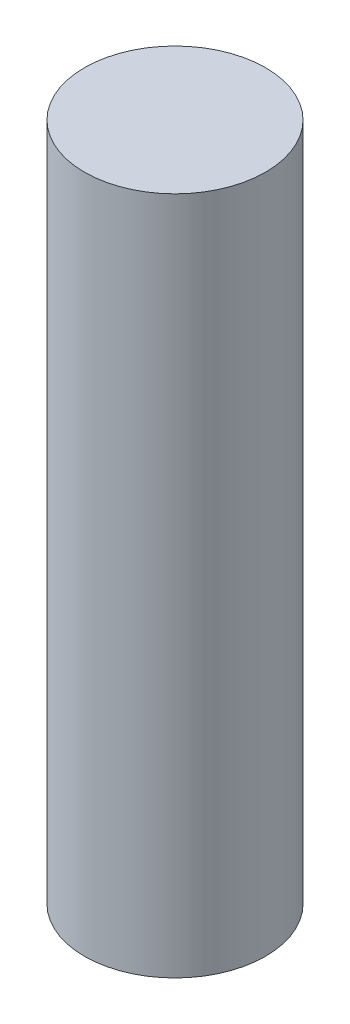
ISO-10303-21;
HEADER;
FILE_DESCRIPTION(('STEP AP214'),'2;1');
FILE_NAME('part.step','',(''),(''),'','','');
FILE_SCHEMA(('AUTOMOTIVE_DESIGN { 1 0 10303 214 1 1 1 1 }'));
ENDSEC;
DATA;
#1=APPLICATION_CONTEXT('core data for automotive mechanical design processes');
#2=APPLICATION_PROTOCOL_DEFINITION('international standard','automotive_design',2000,#1);
#3=PRODUCT_CONTEXT('',#1,'mechanical');
#4=PRODUCT('Part','Part','',(#3));
#5=PRODUCT_RELATED_PRODUCT_CATEGORY('part','',(#4));
#6=PRODUCT_DEFINITION_FORMATION('','',#4);
#7=PRODUCT_DEFINITION_CONTEXT('part definition',#1,'design');
#8=PRODUCT_DEFINITION('design','',#6,#7);
#9=PRODUCT_DEFINITION_SHAPE('','',#8);
#10=(LENGTH_UNIT() NAMED_UNIT(*) SI_UNIT(.MILLI.,.METRE.));
#11=(NAMED_UNIT(*) PLANE_ANGLE_UNIT() SI_UNIT($,.RADIAN.));
#12=(NAMED_UNIT(*) SI_UNIT($,.STERADIAN.) SOLID_ANGLE_UNIT());
#13=UNCERTAINTY_MEASURE_WITH_UNIT(LENGTH_MEASURE(1.E-05),#10,'distance_accuracy_value','');
#14=(GEOMETRIC_REPRESENTATION_CONTEXT(3) GLOBAL_UNCERTAINTY_ASSIGNED_CONTEXT((#13)) GLOBAL_UNIT_ASSIGNED_CONTEXT((#10,
#11,#12)) REPRESENTATION_CONTEXT('',''));
#15=CARTESIAN_POINT('',(0.,0.,0.));
#16=DIRECTION('',(0.,0.,1.));
#17=DIRECTION('',(1.,0.,0.));
#18=AXIS2_PLACEMENT_3D('',#15,#16,#17);
#19=CARTESIAN_POINT('',(0.,22.5,0.));
#20=DIRECTION('',(0.,-1.,0.));
#21=DIRECTION('',(0.,0.,-1.));
#22=AXIS2_PLACEMENT_3D('',#19,#20,#21);
#23=CYLINDRICAL_SURFACE('',#22,6.);
#24=CARTESIAN_POINT('',(0.,22.5,0.));
#25=DIRECTION('',(0.,1.,0.));
#26=DIRECTION('',(0.,0.,1.));
#27=AXIS2_PLACEMENT_3D('',#24,#25,#26);
#28=CIRCLE('',#27,6.);
#29=CARTESIAN_POINT('',(0.,22.5,-6.));
#30=VERTEX_POINT('',#29);
#31=EDGE_CURVE('E10',#30,#30,#28,.T.);
#32=CARTESIAN_POINT('',(0.,-22.5,0.));
#33=DIRECTION('',(0.,1.,0.));
#34=DIRECTION('',(0.,0.,1.));
#35=AXIS2_PLACEMENT_3D('',#32,#33,#34);
#36=CIRCLE('',#35,6.);
#37=CARTESIAN_POINT('',(0.,-22.5,-6.));
#38=VERTEX_POINT('',#37);
#39=EDGE_CURVE('E37',#38,#38,#36,.T.);
#40=CARTESIAN_POINT('',(0.,22.5,-6.));
#41=CARTESIAN_POINT('',(0.,22.03125,-6.));
#42=CARTESIAN_POINT('',(0.,21.5625,-6.));
#43=CARTESIAN_POINT('',(0.,20.625,-6.));
#44=CARTESIAN_POINT('',(0.,20.15625,-6.));
#45=CARTESIAN_POINT('',(0.,19.21875,-6.));
#46=CARTESIAN_POINT('',(0.,18.75,-6.));
#47=CARTESIAN_POINT('',(0.,17.8125,-6.));
#48=CARTESIAN_POINT('',(0.,17.34375,-6.));
#49=CARTESIAN_POINT('',(0.,16.40625,-6.));
#50=CARTESIAN_POINT('',(0.,15.9375,-6.));
#51=CARTESIAN_POINT('',(0.,15.,-6.));
#52=CARTESIAN_POINT('',(0.,14.53125,-6.));
#53=CARTESIAN_POINT('',(0.,13.59375,-6.));
#54=CARTESIAN_POINT('',(0.,13.125,-6.));
#55=CARTESIAN_POINT('',(0.,12.1875,-6.));
#56=CARTESIAN_POINT('',(0.,11.71875,-6.));
#57=CARTESIAN_POINT('',(0.,10.78125,-6.));
#58=CARTESIAN_POINT('',(0.,10.3125,-6.));
#59=CARTESIAN_POINT('',(0.,9.37499999999999,-6.));
#60=CARTESIAN_POINT('',(0.,8.90625,-6.));
#61=CARTESIAN_POINT('',(0.,7.96874999999999,-6.));
#62=CARTESIAN_POINT('',(0.,7.5,-6.));
#63=CARTESIAN_POINT('',(0.,6.5625,-6.));
#64=CARTESIAN_POINT('',(0.,6.09375,-6.));
#65=CARTESIAN_POINT('',(0.,5.15625,-6.));
#66=CARTESIAN_POINT('',(0.,4.6875,-6.));
#67=CARTESIAN_POINT('',(0.,3.75,-6.));
#68=CARTESIAN_POINT('',(0.,3.28125,-6.));
#69=CARTESIAN_POINT('',(0.,2.34375,-6.));
#70=CARTESIAN_POINT('',(0.,1.875,-6.));
#71=CARTESIAN_POINT('',(0.,0.937499999999997,-6.));
#72=CARTESIAN_POINT('',(0.,0.468749999999997,-6.));
#73=CARTESIAN_POINT('',(0.,-0.468750000000004,-6.));
#74=CARTESIAN_POINT('',(0.,-0.937500000000004,-6.));
#75=CARTESIAN_POINT('',(0.,-1.87500000000001,-6.));
#76=CARTESIAN_POINT('',(0.,-2.34375000000001,-6.));
#77=CARTESIAN_POINT('',(0.,-3.28125,-6.));
#78=CARTESIAN_POINT('',(0.,-3.75,-6.));
#79=CARTESIAN_POINT('',(0.,-4.6875,-6.));
#80=CARTESIAN_POINT('',(0.,-5.15625,-6.));
#81=CARTESIAN_POINT('',(0.,-6.09375000000001,-6.));
#82=CARTESIAN_POINT('',(0.,-6.56250000000001,-6.));
#83=CARTESIAN_POINT('',(0.,-7.50000000000001,-6.));
#84=CARTESIAN_POINT('',(0.,-7.96875000000001,-6.));
#85=CARTESIAN_POINT('',(0.,-8.90625,-6.));
#86=CARTESIAN_POINT('',(0.,-9.37500000000001,-6.));
#87=CARTESIAN_POINT('',(0.,-10.3125,-6.));
#88=CARTESIAN_POINT('',(0.,-10.78125,-6.));
#89=CARTESIAN_POINT('',(0.,-11.71875,-6.));
#90=CARTESIAN_POINT('',(0.,-12.1875,-6.));
#91=CARTESIAN_POINT('',(0.,-13.125,-6.));
#92=CARTESIAN_POINT('',(0.,-13.59375,-6.));
#93=CARTESIAN_POINT('',(0.,-14.53125,-6.));
#94=CARTESIAN_POINT('',(0.,-15.,-6.));
#95=CARTESIAN_POINT('',(0.,-15.9375,-6.));
#96=CARTESIAN_POINT('',(0.,-16.40625,-6.));
#97=CARTESIAN_POINT('',(0.,-17.34375,-6.));
#98=CARTESIAN_POINT('',(0.,-17.8125,-6.));
#99=CARTESIAN_POINT('',(0.,-18.75,-6.));
#100=CARTESIAN_POINT('',(0.,-19.21875,-6.));
#101=CARTESIAN_POINT('',(0.,-20.15625,-6.));
#102=CARTESIAN_POINT('',(0.,-20.625,-6.));
#103=CARTESIAN_POINT('',(0.,-21.5625,-6.));
#104=CARTESIAN_POINT('',(0.,-22.03125,-6.));
#105=CARTESIAN_POINT('',(0.,-22.5,-6.));
#106=B_SPLINE_CURVE_WITH_KNOTS('',3,(#40,#41,#42,#43,#44,#45,#46,#47,#48,#49,#50,#51,#52,#53,
#54,#55,#56,#57,#58,#59,#60,#61,#62,#63,#64,#65,#66,#67,#68,#69,#70,#71,#72,#73,#74,#75,#76,#77,
#78,#79,#80,#81,#82,#83,#84,#85,#86,#87,#88,#89,#90,#91,#92,#93,#94,#95,#96,#97,#98,#99,#100,
#101,#102,#103,#104,#105),.UNSPECIFIED.,.F.,.F.,(4,2,2,2,2,2,2,2,2,2,2,2,2,2,2,2,2,2,2,2,2,2,2,
2,2,2,2,2,2,2,2,2,4),(0.,1.40625,2.8125,4.21875,5.625,7.03125,8.4375,9.84375,11.25,12.65625,
14.0625,15.46875,16.875,18.28125,19.6875,21.09375,22.5,23.90625,25.3125,26.71875,28.125,
29.53125,30.9375,32.34375,33.75,35.15625,36.5625,37.96875,39.375,40.78125,42.1875,43.59375,45.),.UNSPECIFIED.);
#107=EDGE_CURVE('BSEAM40',#30,#38,#106,.T.);
#108=ORIENTED_EDGE('',*,*,#31,.F.);
#109=ORIENTED_EDGE('',*,*,#39,.T.);
#110=ORIENTED_EDGE('',*,*,#107,.T.);
#111=ORIENTED_EDGE('',*,*,#107,.F.);
#112=EDGE_LOOP('',(#108,#110,#109,#111));
#113=FACE_BOUND('',#112,.T.);
#114=ADVANCED_FACE('F40',(#113),#23,.T.);
#115=CARTESIAN_POINT('',(0.,22.5,0.));
#116=DIRECTION('',(0.,1.,0.));
#117=DIRECTION('',(0.,0.,1.));
#118=AXIS2_PLACEMENT_3D('',#115,#116,#117);
#119=PLANE('',#118);
#120=ORIENTED_EDGE('',*,*,#31,.T.);
#121=EDGE_LOOP('',(#120));
#122=FACE_BOUND('',#121,.T.);
#123=ADVANCED_FACE('F55',(#122),#119,.T.);
#124=CARTESIAN_POINT('',(0.,-22.5,0.));
#125=DIRECTION('',(0.,1.,0.));
#126=DIRECTION('',(0.,0.,1.));
#127=AXIS2_PLACEMENT_3D('',#124,#125,#126);
#128=PLANE('',#127);
#129=ORIENTED_EDGE('',*,*,#39,.F.);
#130=EDGE_LOOP('',(#129));
#131=FACE_BOUND('',#130,.T.);
#132=ADVANCED_FACE('F49',(#131),#128,.F.);
#133=CLOSED_SHELL('',(#114,#123,#132));
#134=MANIFOLD_SOLID_BREP('B2',#133);
#135=ADVANCED_BREP_SHAPE_REPRESENTATION('',(#18,#134),#14);
#136=SHAPE_DEFINITION_REPRESENTATION(#9,#135);
ENDSEC;
END-ISO-10303-21;
